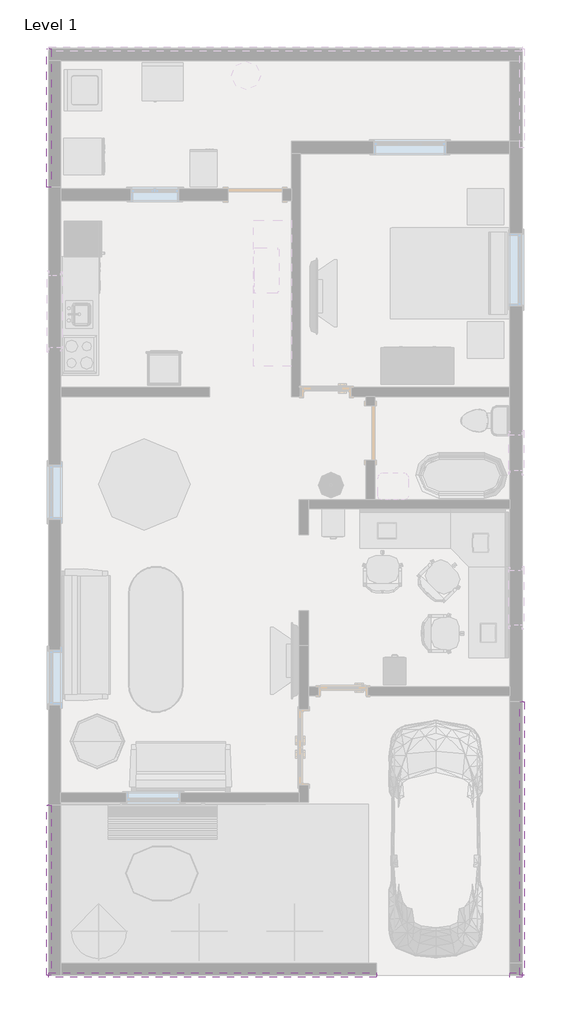
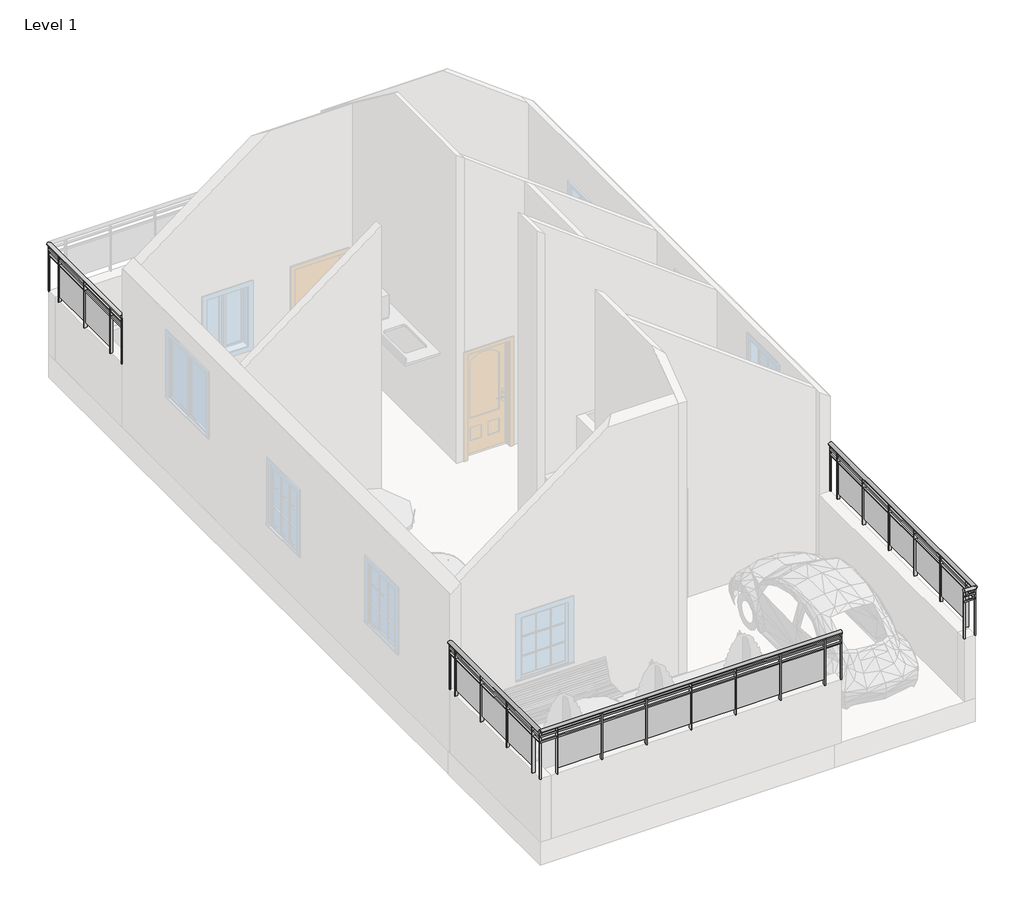
# One storey, part 2 of 3: 5 railings.
"""IFC4 building model written with IfcOpenShell, lengths in millimetres."""

from ifc_helpers import new_model, si_unit, point, frame, origin, place, context, project, spatial, polyline, ellipse_curve, trimmed, outline, extrude, element, save
from ifc_brep_helpers import plane_surface, extruded_surface, advanced_brep

model = new_model("IFC4")

# Units and contexts
model_context = context("Model", 3, world=origin())
ifc_project = project(units=[si_unit("LENGTHUNIT", "METRE", prefix="MILLI")], contexts=[model_context])

# Site, building, storey
site = spatial("IfcSite", under=ifc_project)
building = spatial("IfcBuilding", under=site)
storey = spatial("IfcBuildingStorey", under=building, Name="Level 1", Elevation=0.0)

# Railings
placement = place(None, origin())
element("IfcRailing", 1, ObjectType="Glass Panel - Bottom Fill", at=placement, inside=storey, context=model_context, shape_type="SolidModel", body=[
    advanced_brep(
    [(-8223.1124913, 9548.7394299, 2133.6), (-8146.9124913, 9548.7394299, 2133.6), (-8223.1124913, 11860.1394299, 2133.6), (-8146.9124913, 11860.1394299, 2133.6)],
    [
        (0, 1, ellipse_curve(frame((-8185.0124913, 9548.7394299, 2133.6), z_axis=(0.0, -1.0, 0.0), x_axis=(1.0, 0.0, 0.0)), 38.1, 28.575)),
        (1, 0, ellipse_curve(frame((-8185.0124913, 9548.7394299, 2133.6), z_axis=(0.0, -1.0, 0.0), x_axis=(1.0, 0.0, 0.0)), 38.1, 28.575)),
        (2, 3, ellipse_curve(frame((-8185.0124913, 11860.1394299, 2133.6), z_axis=(0.0, 1.0, 0.0), x_axis=(1.0, 0.0, 0.0)), 38.1, 28.575)),
        (3, 2, ellipse_curve(frame((-8185.0124913, 11860.1394299, 2133.6), z_axis=(0.0, 1.0, 0.0), x_axis=(1.0, 0.0, 0.0)), 38.1, 28.575)),
        (0, 2),
        (3, 1),
    ],
    [
        plane_surface(frame((-8185.0124913, 9548.7394299, 2133.6), z_axis=(0.0, -1.0, 0.0), x_axis=(0.0, 0.0, 1.0))),
        plane_surface(frame((-8185.0124913, 11860.1394299, 2133.6), z_axis=(0.0, 1.0, 0.0), x_axis=(0.0, 0.0, 1.0))),
        extruded_surface(trimmed(ellipse_curve(frame((-8185.0124913, 11860.1394299, 2133.6), z_axis=(0.0, -1.0, 0.0), x_axis=(1.0, 0.0, 0.0)), 38.1, 28.575), [point((-8223.1124913, 11860.1394299, 2133.6))], [point((-8146.9124913, 11860.1394299, 2133.6))], True, "CARTESIAN"), (0.0, -2311.3999999999996, 0.0), 2311.3999999999996),
        extruded_surface(trimmed(ellipse_curve(frame((-8185.0124913, 11860.1394299, 2133.6), z_axis=(0.0, -1.0, 0.0), x_axis=(1.0, 0.0, 0.0)), 38.1, 28.575), [point((-8146.9124913, 11860.1394299, 2133.6))], [point((-8223.1124913, 11860.1394299, 2133.6))], True, "CARTESIAN"), (0.0, -2311.3999999999996, 0.0), 2311.3999999999996),
    ],
    [
        (0, [[1, 2]]),
        (1, [[3, 4]]),
        (2, [[-1, 5, -4, 6]]),
        (3, [[-2, -6, -3, -5]]),
    ],
),
    extrude(outline(polyline([(-8172.3124913, 9548.7394299), (-8197.7124913, 9548.7394299), (-8197.7124913, 11860.1394299), (-8172.3124913, 11860.1394299), (-8172.3124913, 9548.7394299)])), frame((0.0, 0.0, 2019.3), z_axis=(0.0, 0.0, 1.0), x_axis=(1.0, 0.0, 0.0)), (0.0, 0.0, 1.0), 25.4),
    extrude(outline(polyline([(-8172.3124913, 9548.7394299), (-8197.7124913, 9548.7394299), (-8197.7124913, 11860.1394299), (-8172.3124913, 11860.1394299), (-8172.3124913, 9548.7394299)])), frame((0.0, 0.0, 1917.7), z_axis=(0.0, 0.0, 1.0), x_axis=(1.0, 0.0, 0.0)), (0.0, 0.0, 1.0), 25.4),
    extrude(outline(polyline([(-8159.6124913, 11510.8894299), (-8210.4124913, 11510.8894299), (-8210.4124913, 11523.5894299), (-8159.6124913, 11523.5894299), (-8159.6124913, 11510.8894299)])), frame((0.0, 0.0, 1219.2), z_axis=(0.0, 0.0, 1.0), x_axis=(1.0, 0.0, 0.0)), (0.0, 0.0, 1.0), 885.6788223),
    extrude(outline(polyline([(-8191.5476483, 10704.4394299), (-8191.5476483, 11517.2394299), (-8185.1976483, 11517.2394299), (-8185.1976483, 10704.4394299), (-8191.5476483, 10704.4394299)])), frame((0.0, 0.0, 1320.8), z_axis=(0.0, 0.0, 1.0), x_axis=(1.0, 0.0, 0.0)), (0.0, 0.0, 1.0), 596.9),
    extrude(outline(polyline([(-8159.6124913, 10698.0894299), (-8210.4124913, 10698.0894299), (-8210.4124913, 10710.7894299), (-8159.6124913, 10710.7894299), (-8159.6124913, 10698.0894299)])), frame((0.0, 0.0, 1219.2), z_axis=(0.0, 0.0, 1.0), x_axis=(1.0, 0.0, 0.0)), (0.0, 0.0, 1.0), 885.6788223),
    extrude(outline(polyline([(-8191.5476483, 9891.6394299), (-8191.5476483, 10704.4394299), (-8185.1976483, 10704.4394299), (-8185.1976483, 9891.6394299), (-8191.5476483, 9891.6394299)])), frame((0.0, 0.0, 1320.8), z_axis=(0.0, 0.0, 1.0), x_axis=(1.0, 0.0, 0.0)), (0.0, 0.0, 1.0), 596.9),
    extrude(outline(polyline([(-8159.6124913, 9885.2894299), (-8210.4124913, 9885.2894299), (-8210.4124913, 9897.9894299), (-8159.6124913, 9897.9894299), (-8159.6124913, 9885.2894299)])), frame((0.0, 0.0, 1219.2), z_axis=(0.0, 0.0, 1.0), x_axis=(1.0, 0.0, 0.0)), (0.0, 0.0, 1.0), 885.6788223),
    extrude(outline(polyline([(-8175.4874913, 11847.4394299), (-8194.5374913, 11847.4394299), (-8194.5374913, 11866.4894299), (-8175.4874913, 11866.4894299), (-8175.4874913, 11847.4394299)])), frame((0.0, 0.0, 1219.2), z_axis=(0.0, 0.0, 1.0), x_axis=(1.0, 0.0, 0.0)), (0.0, 0.0, 1.0), 885.6788223),
    extrude(outline(polyline([(-8175.4874913, 9542.3894299), (-8194.5374913, 9542.3894299), (-8194.5374913, 9561.4394299), (-8175.4874913, 9561.4394299), (-8175.4874913, 9542.3894299)])), frame((0.0, 0.0, 1219.2), z_axis=(0.0, 0.0, 1.0), x_axis=(1.0, 0.0, 0.0)), (0.0, 0.0, 1.0), 885.6788223),
])
element("IfcRailing", 2, ObjectType="Glass Panel - Bottom Fill", at=placement, inside=storey, context=model_context, shape_type="SolidModel", body=[
    advanced_brep(
    [(-8146.9124913, -789.0605701, 2133.6), (-8223.1124913, -789.0605701, 2133.6), (-8146.9124913, -3633.8605701, 2133.6), (-8223.1124913, -3633.8605701, 2133.6)],
    [
        (0, 1, ellipse_curve(frame((-8185.0124913, -789.0605701, 2133.6), z_axis=(0.0, 1.0, 0.0), x_axis=(-1.0, 0.0, 0.0)), 38.1, 28.575)),
        (1, 0, ellipse_curve(frame((-8185.0124913, -789.0605701, 2133.6), z_axis=(0.0, 1.0, 0.0), x_axis=(-1.0, 0.0, 0.0)), 38.1, 28.575)),
        (2, 3, ellipse_curve(frame((-8185.0124913, -3633.8605701, 2133.6), z_axis=(0.0, -1.0, 0.0), x_axis=(-1.0, 0.0, 0.0)), 38.1, 28.575)),
        (3, 2, ellipse_curve(frame((-8185.0124913, -3633.8605701, 2133.6), z_axis=(0.0, -1.0, 0.0), x_axis=(-1.0, 0.0, 0.0)), 38.1, 28.575)),
        (0, 2),
        (3, 1),
    ],
    [
        plane_surface(frame((-8185.0124913, -789.0605701, 2133.6), z_axis=(0.0, 1.0, 0.0), x_axis=(0.0, 0.0, -1.0))),
        plane_surface(frame((-8185.0124913, -3633.8605701, 2133.6), z_axis=(0.0, -1.0, 0.0), x_axis=(0.0, 0.0, -1.0))),
        extruded_surface(trimmed(ellipse_curve(frame((-8185.0124913, -3633.8605701, 2133.6), z_axis=(0.0, 1.0, 0.0), x_axis=(-1.0, 0.0, 0.0)), 38.1, 28.575), [point((-8146.9124913, -3633.8605701, 2133.6))], [point((-8223.1124913, -3633.8605701, 2133.6))], True, "CARTESIAN"), (0.0, 2844.8, 0.0), 2844.8),
        extruded_surface(trimmed(ellipse_curve(frame((-8185.0124913, -3633.8605701, 2133.6), z_axis=(0.0, 1.0, 0.0), x_axis=(-1.0, 0.0, 0.0)), 38.1, 28.575), [point((-8223.1124913, -3633.8605701, 2133.6))], [point((-8146.9124913, -3633.8605701, 2133.6))], True, "CARTESIAN"), (0.0, 2844.8, 0.0), 2844.8),
    ],
    [
        (0, [[1, 2]]),
        (1, [[3, 4]]),
        (2, [[-1, 5, -4, 6]]),
        (3, [[-2, -6, -3, -5]]),
    ],
),
    extrude(outline(polyline([(-8197.7124913, -789.0605701), (-8172.3124913, -789.0605701), (-8172.3124913, -3633.8605701), (-8197.7124913, -3633.8605701), (-8197.7124913, -789.0605701)])), frame((0.0, 0.0, 2019.3), z_axis=(0.0, 0.0, 1.0), x_axis=(1.0, 0.0, 0.0)), (0.0, 0.0, 1.0), 25.4),
    extrude(outline(polyline([(-8197.7124913, -789.0605701), (-8172.3124913, -789.0605701), (-8172.3124913, -3633.8605701), (-8197.7124913, -3633.8605701), (-8197.7124913, -789.0605701)])), frame((0.0, 0.0, 1917.7), z_axis=(0.0, 0.0, 1.0), x_axis=(1.0, 0.0, 0.0)), (0.0, 0.0, 1.0), 25.4),
    extrude(outline(polyline([(-8210.4124913, -3424.3105701), (-8159.6124913, -3424.3105701), (-8159.6124913, -3437.0105701), (-8210.4124913, -3437.0105701), (-8210.4124913, -3424.3105701)])), frame((0.0, 0.0, 1219.2), z_axis=(0.0, 0.0, 1.0), x_axis=(1.0, 0.0, 0.0)), (0.0, 0.0, 1.0), 885.6788223),
    extrude(outline(polyline([(-8178.4773343, -2617.8605701), (-8178.4773343, -3430.6605701), (-8184.8273343, -3430.6605701), (-8184.8273343, -2617.8605701), (-8178.4773343, -2617.8605701)])), frame((0.0, 0.0, 1320.8), z_axis=(0.0, 0.0, 1.0), x_axis=(1.0, 0.0, 0.0)), (0.0, 0.0, 1.0), 596.9),
    extrude(outline(polyline([(-8210.4124913, -2611.5105701), (-8159.6124913, -2611.5105701), (-8159.6124913, -2624.2105701), (-8210.4124913, -2624.2105701), (-8210.4124913, -2611.5105701)])), frame((0.0, 0.0, 1219.2), z_axis=(0.0, 0.0, 1.0), x_axis=(1.0, 0.0, 0.0)), (0.0, 0.0, 1.0), 885.6788223),
    extrude(outline(polyline([(-8178.4773343, -1805.0605701), (-8178.4773343, -2617.8605701), (-8184.8273343, -2617.8605701), (-8184.8273343, -1805.0605701), (-8178.4773343, -1805.0605701)])), frame((0.0, 0.0, 1320.8), z_axis=(0.0, 0.0, 1.0), x_axis=(1.0, 0.0, 0.0)), (0.0, 0.0, 1.0), 596.9),
    extrude(outline(polyline([(-8210.4124913, -1798.7105701), (-8159.6124913, -1798.7105701), (-8159.6124913, -1811.4105701), (-8210.4124913, -1811.4105701), (-8210.4124913, -1798.7105701)])), frame((0.0, 0.0, 1219.2), z_axis=(0.0, 0.0, 1.0), x_axis=(1.0, 0.0, 0.0)), (0.0, 0.0, 1.0), 885.6788223),
    extrude(outline(polyline([(-8178.4773343, -992.2605701), (-8178.4773343, -1805.0605701), (-8184.8273343, -1805.0605701), (-8184.8273343, -992.2605701), (-8178.4773343, -992.2605701)])), frame((0.0, 0.0, 1320.8), z_axis=(0.0, 0.0, 1.0), x_axis=(1.0, 0.0, 0.0)), (0.0, 0.0, 1.0), 596.9),
    extrude(outline(polyline([(-8210.4124913, -985.9105701), (-8159.6124913, -985.9105701), (-8159.6124913, -998.6105701), (-8210.4124913, -998.6105701), (-8210.4124913, -985.9105701)])), frame((0.0, 0.0, 1219.2), z_axis=(0.0, 0.0, 1.0), x_axis=(1.0, 0.0, 0.0)), (0.0, 0.0, 1.0), 885.6788223),
    extrude(outline(polyline([(-8194.5374913, -3621.1605701), (-8175.4874913, -3621.1605701), (-8175.4874913, -3640.2105701), (-8194.5374913, -3640.2105701), (-8194.5374913, -3621.1605701)])), frame((0.0, 0.0, 1219.2), z_axis=(0.0, 0.0, 1.0), x_axis=(1.0, 0.0, 0.0)), (0.0, 0.0, 1.0), 885.6788223),
    extrude(outline(polyline([(-8194.5374913, -782.7105701), (-8175.4874913, -782.7105701), (-8175.4874913, -801.7605701), (-8194.5374913, -801.7605701), (-8194.5374913, -782.7105701)])), frame((0.0, 0.0, 1219.2), z_axis=(0.0, 0.0, 1.0), x_axis=(1.0, 0.0, 0.0)), (0.0, 0.0, 1.0), 885.6788223),
])
element("IfcRailing", 3, ObjectType="Glass Panel - Bottom Fill", at=placement, inside=storey, context=model_context, shape_type="SolidModel", body=[
    advanced_brep(
    [(-8185.0124913, -3595.7605701, 2133.6), (-8185.0124913, -3671.9605701, 2133.6), (-2698.6124913, -3595.7605701, 2133.6), (-2698.6124913, -3671.9605701, 2133.6)],
    [
        (0, 1, ellipse_curve(frame((-8185.0124913, -3633.8605701, 2133.6), z_axis=(-1.0, 0.0, 0.0), x_axis=(0.0, -1.0, 0.0)), 38.1, 28.575)),
        (1, 0, ellipse_curve(frame((-8185.0124913, -3633.8605701, 2133.6), z_axis=(-1.0, 0.0, 0.0), x_axis=(0.0, -1.0, 0.0)), 38.1, 28.575)),
        (2, 3, ellipse_curve(frame((-2698.6124913, -3633.8605701, 2133.6), z_axis=(1.0, 0.0, 0.0), x_axis=(0.0, -1.0, 0.0)), 38.1, 28.575)),
        (3, 2, ellipse_curve(frame((-2698.6124913, -3633.8605701, 2133.6), z_axis=(1.0, 0.0, 0.0), x_axis=(0.0, -1.0, 0.0)), 38.1, 28.575)),
        (0, 2),
        (3, 1),
    ],
    [
        plane_surface(frame((-8185.0124913, -3633.8605701, 2133.6), z_axis=(-1.0, 0.0, 0.0), x_axis=(0.0, 1.0, 0.0))),
        plane_surface(frame((-2698.6124913, -3633.8605701, 2133.6), z_axis=(1.0, 0.0, 0.0), x_axis=(0.0, 1.0, 0.0))),
        extruded_surface(trimmed(ellipse_curve(frame((-2698.6124913, -3633.8605701, 2133.6), z_axis=(-1.0, 0.0, 0.0), x_axis=(0.0, -1.0, 0.0)), 38.1, 28.575), [point((-2698.6124913, -3595.7605701, 2133.6))], [point((-2698.6124913, -3671.9605701, 2133.6))], True, "CARTESIAN"), (-5486.4, 0.0, 0.0), 5486.4),
        extruded_surface(trimmed(ellipse_curve(frame((-2698.6124913, -3633.8605701, 2133.6), z_axis=(-1.0, 0.0, 0.0), x_axis=(0.0, -1.0, 0.0)), 38.1, 28.575), [point((-2698.6124913, -3671.9605701, 2133.6))], [point((-2698.6124913, -3595.7605701, 2133.6))], True, "CARTESIAN"), (-5486.4, 0.0, 0.0), 5486.4),
    ],
    [
        (0, [[1, 2]]),
        (1, [[3, 4]]),
        (2, [[-1, 5, -4, 6]]),
        (3, [[-2, -6, -3, -5]]),
    ],
),
    extrude(outline(polyline([(-8185.0124913, -3646.5605701), (-8185.0124913, -3621.1605701), (-2698.6124913, -3621.1605701), (-2698.6124913, -3646.5605701), (-8185.0124913, -3646.5605701)])), frame((0.0, 0.0, 2019.3), z_axis=(0.0, 0.0, 1.0), x_axis=(1.0, 0.0, 0.0)), (0.0, 0.0, 1.0), 25.4),
    extrude(outline(polyline([(-8185.0124913, -3646.5605701), (-8185.0124913, -3621.1605701), (-2698.6124913, -3621.1605701), (-2698.6124913, -3646.5605701), (-8185.0124913, -3646.5605701)])), frame((0.0, 0.0, 1917.7), z_axis=(0.0, 0.0, 1.0), x_axis=(1.0, 0.0, 0.0)), (0.0, 0.0, 1.0), 25.4),
    extrude(outline(polyline([(-3009.7624913, -3659.2605701), (-3009.7624913, -3608.4605701), (-2997.0624913, -3608.4605701), (-2997.0624913, -3659.2605701), (-3009.7624913, -3659.2605701)])), frame((0.0, 0.0, 1219.2), z_axis=(0.0, 0.0, 1.0), x_axis=(1.0, 0.0, 0.0)), (0.0, 0.0, 1.0), 885.6788223),
    extrude(outline(polyline([(-3816.2124913, -3627.3254131), (-3003.4124913, -3627.3254131), (-3003.4124913, -3633.6754131), (-3816.2124913, -3633.6754131), (-3816.2124913, -3627.3254131)])), frame((0.0, 0.0, 1320.8), z_axis=(0.0, 0.0, 1.0), x_axis=(1.0, 0.0, 0.0)), (0.0, 0.0, 1.0), 596.9),
    extrude(outline(polyline([(-3822.5624913, -3659.2605701), (-3822.5624913, -3608.4605701), (-3809.8624913, -3608.4605701), (-3809.8624913, -3659.2605701), (-3822.5624913, -3659.2605701)])), frame((0.0, 0.0, 1219.2), z_axis=(0.0, 0.0, 1.0), x_axis=(1.0, 0.0, 0.0)), (0.0, 0.0, 1.0), 885.6788223),
    extrude(outline(polyline([(-4629.0124913, -3627.3254131), (-3816.2124913, -3627.3254131), (-3816.2124913, -3633.6754131), (-4629.0124913, -3633.6754131), (-4629.0124913, -3627.3254131)])), frame((0.0, 0.0, 1320.8), z_axis=(0.0, 0.0, 1.0), x_axis=(1.0, 0.0, 0.0)), (0.0, 0.0, 1.0), 596.9),
    extrude(outline(polyline([(-4635.3624913, -3659.2605701), (-4635.3624913, -3608.4605701), (-4622.6624913, -3608.4605701), (-4622.6624913, -3659.2605701), (-4635.3624913, -3659.2605701)])), frame((0.0, 0.0, 1219.2), z_axis=(0.0, 0.0, 1.0), x_axis=(1.0, 0.0, 0.0)), (0.0, 0.0, 1.0), 885.6788223),
    extrude(outline(polyline([(-5441.8124913, -3627.3254131), (-4629.0124913, -3627.3254131), (-4629.0124913, -3633.6754131), (-5441.8124913, -3633.6754131), (-5441.8124913, -3627.3254131)])), frame((0.0, 0.0, 1320.8), z_axis=(0.0, 0.0, 1.0), x_axis=(1.0, 0.0, 0.0)), (0.0, 0.0, 1.0), 596.9),
    extrude(outline(polyline([(-5448.1624913, -3659.2605701), (-5448.1624913, -3608.4605701), (-5435.4624913, -3608.4605701), (-5435.4624913, -3659.2605701), (-5448.1624913, -3659.2605701)])), frame((0.0, 0.0, 1219.2), z_axis=(0.0, 0.0, 1.0), x_axis=(1.0, 0.0, 0.0)), (0.0, 0.0, 1.0), 885.6788223),
    extrude(outline(polyline([(-6254.6124913, -3627.3254131), (-5441.8124913, -3627.3254131), (-5441.8124913, -3633.6754131), (-6254.6124913, -3633.6754131), (-6254.6124913, -3627.3254131)])), frame((0.0, 0.0, 1320.8), z_axis=(0.0, 0.0, 1.0), x_axis=(1.0, 0.0, 0.0)), (0.0, 0.0, 1.0), 596.9),
    extrude(outline(polyline([(-6260.9624913, -3659.2605701), (-6260.9624913, -3608.4605701), (-6248.2624913, -3608.4605701), (-6248.2624913, -3659.2605701), (-6260.9624913, -3659.2605701)])), frame((0.0, 0.0, 1219.2), z_axis=(0.0, 0.0, 1.0), x_axis=(1.0, 0.0, 0.0)), (0.0, 0.0, 1.0), 885.6788223),
    extrude(outline(polyline([(-7067.4124913, -3627.3254131), (-6254.6124913, -3627.3254131), (-6254.6124913, -3633.6754131), (-7067.4124913, -3633.6754131), (-7067.4124913, -3627.3254131)])), frame((0.0, 0.0, 1320.8), z_axis=(0.0, 0.0, 1.0), x_axis=(1.0, 0.0, 0.0)), (0.0, 0.0, 1.0), 596.9),
    extrude(outline(polyline([(-7073.7624913, -3659.2605701), (-7073.7624913, -3608.4605701), (-7061.0624913, -3608.4605701), (-7061.0624913, -3659.2605701), (-7073.7624913, -3659.2605701)])), frame((0.0, 0.0, 1219.2), z_axis=(0.0, 0.0, 1.0), x_axis=(1.0, 0.0, 0.0)), (0.0, 0.0, 1.0), 885.6788223),
    extrude(outline(polyline([(-7880.2124913, -3627.3254131), (-7067.4124913, -3627.3254131), (-7067.4124913, -3633.6754131), (-7880.2124913, -3633.6754131), (-7880.2124913, -3627.3254131)])), frame((0.0, 0.0, 1320.8), z_axis=(0.0, 0.0, 1.0), x_axis=(1.0, 0.0, 0.0)), (0.0, 0.0, 1.0), 596.9),
    extrude(outline(polyline([(-7886.5624913, -3659.2605701), (-7886.5624913, -3608.4605701), (-7873.8624913, -3608.4605701), (-7873.8624913, -3659.2605701), (-7886.5624913, -3659.2605701)])), frame((0.0, 0.0, 1219.2), z_axis=(0.0, 0.0, 1.0), x_axis=(1.0, 0.0, 0.0)), (0.0, 0.0, 1.0), 885.6788223),
    extrude(outline(polyline([(-2711.3124913, -3643.3855701), (-2711.3124913, -3624.3355701), (-2692.2624913, -3624.3355701), (-2692.2624913, -3643.3855701), (-2711.3124913, -3643.3855701)])), frame((0.0, 0.0, 1219.2), z_axis=(0.0, 0.0, 1.0), x_axis=(1.0, 0.0, 0.0)), (0.0, 0.0, 1.0), 885.6788223),
    extrude(outline(polyline([(-8191.3624913, -3643.3855701), (-8191.3624913, -3624.3355701), (-8172.3124913, -3624.3355701), (-8172.3124913, -3643.3855701), (-8191.3624913, -3643.3855701)])), frame((0.0, 0.0, 1219.2), z_axis=(0.0, 0.0, 1.0), x_axis=(1.0, 0.0, 0.0)), (0.0, 0.0, 1.0), 885.6788223),
])
element("IfcRailing", 4, ObjectType="Glass Panel - Bottom Fill", at=placement, inside=storey, context=model_context, shape_type="SolidModel", body=[
    advanced_brep(
    [(-463.4124913, -3595.7605701, 2133.6), (-463.4124913, -3671.9605701, 2133.6), (-260.2124913, -3595.7605701, 2133.6), (-260.2124913, -3671.9605701, 2133.6)],
    [
        (0, 1, ellipse_curve(frame((-463.4124913, -3633.8605701, 2133.6), z_axis=(-1.0, 0.0, 0.0), x_axis=(0.0, -1.0, 0.0)), 38.1, 28.575)),
        (1, 0, ellipse_curve(frame((-463.4124913, -3633.8605701, 2133.6), z_axis=(-1.0, 0.0, 0.0), x_axis=(0.0, -1.0, 0.0)), 38.1, 28.575)),
        (2, 3, ellipse_curve(frame((-260.2124913, -3633.8605701, 2133.6), z_axis=(1.0, 0.0, 0.0), x_axis=(0.0, -1.0, 0.0)), 38.1, 28.575)),
        (3, 2, ellipse_curve(frame((-260.2124913, -3633.8605701, 2133.6), z_axis=(1.0, 0.0, 0.0), x_axis=(0.0, -1.0, 0.0)), 38.1, 28.575)),
        (0, 2),
        (3, 1),
    ],
    [
        plane_surface(frame((-463.4124913, -3633.8605701, 2133.6), z_axis=(-1.0, 0.0, 0.0), x_axis=(0.0, 1.0, 0.0))),
        plane_surface(frame((-260.2124913, -3633.8605701, 2133.6), z_axis=(1.0, 0.0, 0.0), x_axis=(0.0, 1.0, 0.0))),
        extruded_surface(trimmed(ellipse_curve(frame((-260.2124913, -3633.8605701, 2133.6), z_axis=(-1.0, 0.0, 0.0), x_axis=(0.0, -1.0, 0.0)), 38.1, 28.575), [point((-260.2124913, -3595.7605701, 2133.6))], [point((-260.2124913, -3671.9605701, 2133.6))], True, "CARTESIAN"), (-203.2, 0.0, 0.0), 203.2),
        extruded_surface(trimmed(ellipse_curve(frame((-260.2124913, -3633.8605701, 2133.6), z_axis=(-1.0, 0.0, 0.0), x_axis=(0.0, -1.0, 0.0)), 38.1, 28.575), [point((-260.2124913, -3671.9605701, 2133.6))], [point((-260.2124913, -3595.7605701, 2133.6))], True, "CARTESIAN"), (-203.2, 0.0, 0.0), 203.2),
    ],
    [
        (0, [[1, 2]]),
        (1, [[3, 4]]),
        (2, [[-1, 5, -4, 6]]),
        (3, [[-2, -6, -3, -5]]),
    ],
),
    extrude(outline(polyline([(-463.4124913, -3646.5605701), (-463.4124913, -3621.1605701), (-260.2124913, -3621.1605701), (-260.2124913, -3646.5605701), (-463.4124913, -3646.5605701)])), frame((0.0, 0.0, 2019.3), z_axis=(0.0, 0.0, 1.0), x_axis=(1.0, 0.0, 0.0)), (0.0, 0.0, 1.0), 25.4),
    extrude(outline(polyline([(-463.4124913, -3646.5605701), (-463.4124913, -3621.1605701), (-260.2124913, -3621.1605701), (-260.2124913, -3646.5605701), (-463.4124913, -3646.5605701)])), frame((0.0, 0.0, 1917.7), z_axis=(0.0, 0.0, 1.0), x_axis=(1.0, 0.0, 0.0)), (0.0, 0.0, 1.0), 25.4),
    extrude(outline(polyline([(-272.9124913, -3643.3855701), (-272.9124913, -3624.3355701), (-253.8624913, -3624.3355701), (-253.8624913, -3643.3855701), (-272.9124913, -3643.3855701)])), frame((0.0, 0.0, 1219.2), z_axis=(0.0, 0.0, 1.0), x_axis=(1.0, 0.0, 0.0)), (0.0, 0.0, 1.0), 885.6788223),
    extrude(outline(polyline([(-469.7624913, -3643.3855701), (-469.7624913, -3624.3355701), (-450.7124913, -3624.3355701), (-450.7124913, -3643.3855701), (-469.7624913, -3643.3855701)])), frame((0.0, 0.0, 1219.2), z_axis=(0.0, 0.0, 1.0), x_axis=(1.0, 0.0, 0.0)), (0.0, 0.0, 1.0), 885.6788223),
])
element("IfcRailing", 5, ObjectType="Glass Panel - Bottom Fill", at=placement, inside=storey, context=model_context, shape_type="SolidModel", body=[
    advanced_brep(
    [(-222.1124913, 938.1394299, 2133.6), (-298.3124913, 938.1394299, 2133.6), (-222.1124913, -3633.8605701, 2133.6), (-298.3124913, -3633.8605701, 2133.6)],
    [
        (0, 1, ellipse_curve(frame((-260.2124913, 938.1394299, 2133.6), z_axis=(0.0, 1.0, 0.0), x_axis=(-1.0, 0.0, 0.0)), 38.1, 28.575)),
        (1, 0, ellipse_curve(frame((-260.2124913, 938.1394299, 2133.6), z_axis=(0.0, 1.0, 0.0), x_axis=(-1.0, 0.0, 0.0)), 38.1, 28.575)),
        (2, 3, ellipse_curve(frame((-260.2124913, -3633.8605701, 2133.6), z_axis=(0.0, -1.0, 0.0), x_axis=(-1.0, 0.0, 0.0)), 38.1, 28.575)),
        (3, 2, ellipse_curve(frame((-260.2124913, -3633.8605701, 2133.6), z_axis=(0.0, -1.0, 0.0), x_axis=(-1.0, 0.0, 0.0)), 38.1, 28.575)),
        (0, 2),
        (3, 1),
    ],
    [
        plane_surface(frame((-260.2124913, 938.1394299, 2133.6), z_axis=(0.0, 1.0, 0.0), x_axis=(0.0, 0.0, -1.0))),
        plane_surface(frame((-260.2124913, -3633.8605701, 2133.6), z_axis=(0.0, -1.0, 0.0), x_axis=(0.0, 0.0, -1.0))),
        extruded_surface(trimmed(ellipse_curve(frame((-260.2124913, -3633.8605701, 2133.6), z_axis=(0.0, 1.0, 0.0), x_axis=(-1.0, 0.0, 0.0)), 38.1, 28.575), [point((-222.1124913, -3633.8605701, 2133.6))], [point((-298.3124913, -3633.8605701, 2133.6))], True, "CARTESIAN"), (0.0, 4572.0, 0.0), 4572.0),
        extruded_surface(trimmed(ellipse_curve(frame((-260.2124913, -3633.8605701, 2133.6), z_axis=(0.0, 1.0, 0.0), x_axis=(-1.0, 0.0, 0.0)), 38.1, 28.575), [point((-298.3124913, -3633.8605701, 2133.6))], [point((-222.1124913, -3633.8605701, 2133.6))], True, "CARTESIAN"), (0.0, 4572.0, 0.0), 4572.0),
    ],
    [
        (0, [[1, 2]]),
        (1, [[3, 4]]),
        (2, [[-1, 5, -4, 6]]),
        (3, [[-2, -6, -3, -5]]),
    ],
),
    extrude(outline(polyline([(-272.9124913, 938.1394299), (-247.5124913, 938.1394299), (-247.5124913, -3633.8605701), (-272.9124913, -3633.8605701), (-272.9124913, 938.1394299)])), frame((0.0, 0.0, 2019.3), z_axis=(0.0, 0.0, 1.0), x_axis=(1.0, 0.0, 0.0)), (0.0, 0.0, 1.0), 25.4),
    extrude(outline(polyline([(-272.9124913, 938.1394299), (-247.5124913, 938.1394299), (-247.5124913, -3633.8605701), (-272.9124913, -3633.8605701), (-272.9124913, 938.1394299)])), frame((0.0, 0.0, 1917.7), z_axis=(0.0, 0.0, 1.0), x_axis=(1.0, 0.0, 0.0)), (0.0, 0.0, 1.0), 25.4),
    extrude(outline(polyline([(-285.6124913, -3373.5105701), (-234.8124913, -3373.5105701), (-234.8124913, -3386.2105701), (-285.6124913, -3386.2105701), (-285.6124913, -3373.5105701)])), frame((0.0, 0.0, 1219.2), z_axis=(0.0, 0.0, 1.0), x_axis=(1.0, 0.0, 0.0)), (0.0, 0.0, 1.0), 885.6788223),
    extrude(outline(polyline([(-253.6773343, -2567.0605701), (-253.6773343, -3379.8605701), (-260.0273343, -3379.8605701), (-260.0273343, -2567.0605701), (-253.6773343, -2567.0605701)])), frame((0.0, 0.0, 1320.8), z_axis=(0.0, 0.0, 1.0), x_axis=(1.0, 0.0, 0.0)), (0.0, 0.0, 1.0), 596.9),
    extrude(outline(polyline([(-285.6124913, -2560.7105701), (-234.8124913, -2560.7105701), (-234.8124913, -2573.4105701), (-285.6124913, -2573.4105701), (-285.6124913, -2560.7105701)])), frame((0.0, 0.0, 1219.2), z_axis=(0.0, 0.0, 1.0), x_axis=(1.0, 0.0, 0.0)), (0.0, 0.0, 1.0), 885.6788223),
    extrude(outline(polyline([(-253.6773343, -1754.2605701), (-253.6773343, -2567.0605701), (-260.0273343, -2567.0605701), (-260.0273343, -1754.2605701), (-253.6773343, -1754.2605701)])), frame((0.0, 0.0, 1320.8), z_axis=(0.0, 0.0, 1.0), x_axis=(1.0, 0.0, 0.0)), (0.0, 0.0, 1.0), 596.9),
    extrude(outline(polyline([(-285.6124913, -1747.9105701), (-234.8124913, -1747.9105701), (-234.8124913, -1760.6105701), (-285.6124913, -1760.6105701), (-285.6124913, -1747.9105701)])), frame((0.0, 0.0, 1219.2), z_axis=(0.0, 0.0, 1.0), x_axis=(1.0, 0.0, 0.0)), (0.0, 0.0, 1.0), 885.6788223),
    extrude(outline(polyline([(-253.6773343, -941.4605701), (-253.6773343, -1754.2605701), (-260.0273343, -1754.2605701), (-260.0273343, -941.4605701), (-253.6773343, -941.4605701)])), frame((0.0, 0.0, 1320.8), z_axis=(0.0, 0.0, 1.0), x_axis=(1.0, 0.0, 0.0)), (0.0, 0.0, 1.0), 596.9),
    extrude(outline(polyline([(-285.6124913, -935.1105701), (-234.8124913, -935.1105701), (-234.8124913, -947.8105701), (-285.6124913, -947.8105701), (-285.6124913, -935.1105701)])), frame((0.0, 0.0, 1219.2), z_axis=(0.0, 0.0, 1.0), x_axis=(1.0, 0.0, 0.0)), (0.0, 0.0, 1.0), 885.6788223),
    extrude(outline(polyline([(-253.6773343, -128.6605701), (-253.6773343, -941.4605701), (-260.0273343, -941.4605701), (-260.0273343, -128.6605701), (-253.6773343, -128.6605701)])), frame((0.0, 0.0, 1320.8), z_axis=(0.0, 0.0, 1.0), x_axis=(1.0, 0.0, 0.0)), (0.0, 0.0, 1.0), 596.9),
    extrude(outline(polyline([(-285.6124913, -122.3105701), (-234.8124913, -122.3105701), (-234.8124913, -135.0105701), (-285.6124913, -135.0105701), (-285.6124913, -122.3105701)])), frame((0.0, 0.0, 1219.2), z_axis=(0.0, 0.0, 1.0), x_axis=(1.0, 0.0, 0.0)), (0.0, 0.0, 1.0), 885.6788223),
    extrude(outline(polyline([(-253.6773343, 684.1394299), (-253.6773343, -128.6605701), (-260.0273343, -128.6605701), (-260.0273343, 684.1394299), (-253.6773343, 684.1394299)])), frame((0.0, 0.0, 1320.8), z_axis=(0.0, 0.0, 1.0), x_axis=(1.0, 0.0, 0.0)), (0.0, 0.0, 1.0), 596.9),
    extrude(outline(polyline([(-285.6124913, 690.4894299), (-234.8124913, 690.4894299), (-234.8124913, 677.7894299), (-285.6124913, 677.7894299), (-285.6124913, 690.4894299)])), frame((0.0, 0.0, 1219.2), z_axis=(0.0, 0.0, 1.0), x_axis=(1.0, 0.0, 0.0)), (0.0, 0.0, 1.0), 885.6788223),
    extrude(outline(polyline([(-269.7374913, -3621.1605701), (-250.6874913, -3621.1605701), (-250.6874913, -3640.2105701), (-269.7374913, -3640.2105701), (-269.7374913, -3621.1605701)])), frame((0.0, 0.0, 1219.2), z_axis=(0.0, 0.0, 1.0), x_axis=(1.0, 0.0, 0.0)), (0.0, 0.0, 1.0), 885.6788223),
    extrude(outline(polyline([(-269.7374913, 944.4894299), (-250.6874913, 944.4894299), (-250.6874913, 925.4394299), (-269.7374913, 925.4394299), (-269.7374913, 944.4894299)])), frame((0.0, 0.0, 1219.2), z_axis=(0.0, 0.0, 1.0), x_axis=(1.0, 0.0, 0.0)), (0.0, 0.0, 1.0), 885.6788223),
])

save(model, "model.ifc")

# Revit data of these elements
# Type "Glass Panel - Bottom Fill"
#   Assembly Code = "C2010400"
#   built-in parameter 1008612 = 0.0416667 (stored number, unit not read)
#   built-in parameter 1008611 = 0.0416667 (stored number, unit not read)
#   built-in parameter 1008609 = 0.333333 (stored number, unit not read)
#   built-in parameter 1008604 = 0.166667 (stored number, unit not read)
#   built-in parameter 1008603 = 0.166667 (stored number, unit not read)
#   Railing Height = 3' - 0"
#   built-in parameter 1008630 = 2
#   built-in parameter 1008610 = 2
#   built-in parameter 1008618 = Baluster - Square : 3/4"
# Elements 1, 2, 3, 5 (IfcRailing, "Glass Panel - Bottom Fill")
#   built-in parameter 1008621 = 4 (stored number, unit not read)
#   Phase Created = New Construction
#   Materials on its faces: "Glass"
# Element 4 (IfcRailing, "Glass Panel - Bottom Fill")
#   built-in parameter 1008621 = 4 (stored number, unit not read)
#   Phase Created = New Construction
# Materials
#   "Glass": class "Glass", colour RGB 0 128 192, transparency 0.75, Description = "Soda Lime Glass", Cost = 0
